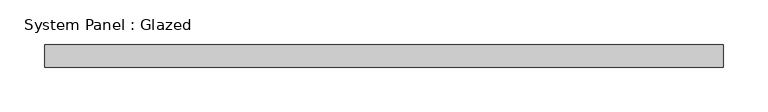
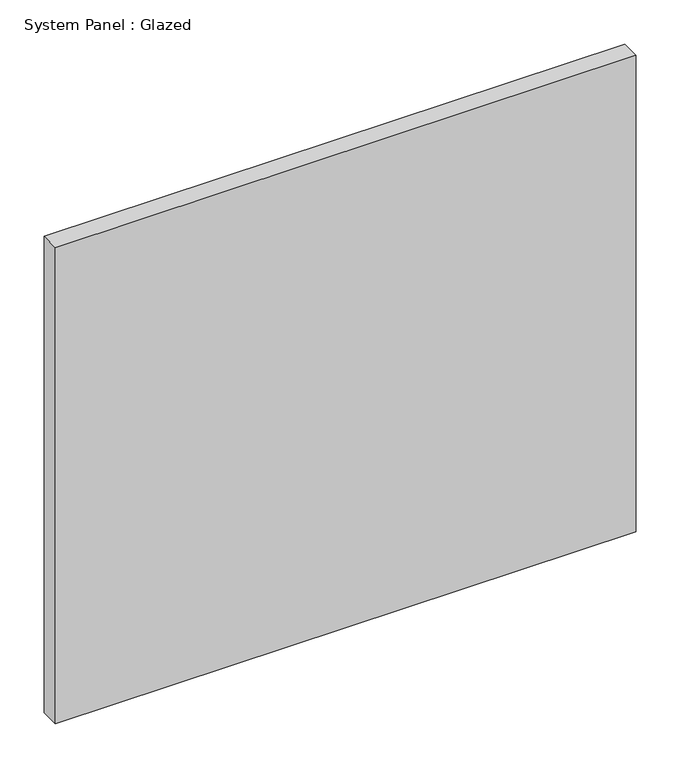
"""IFC4 building model written with IfcOpenShell, lengths in millimetres: plate geometry, System Panel : Glazed."""

from ifc_helpers import new_model, si_unit, origin, origin_with_axes, place, context, project, spatial, polyline, outline, extrude, source, transform, mapped, element, save


def system_panel_glazed_55f8bac4(model_context):
    return source(origin(), model_context, "Body", "SweptSolid", [
        extrude(outline(polyline([(381.0, 19.05), (-381.0, 19.05), (-381.0, 44.45), (381.0, 44.45), (381.0, 19.05)])), origin_with_axes(), (0.0, 0.0, 1.0), 660.4),
    ])


if __name__ == "__main__":
    model = new_model("IFC4")
    model_context = context("Model", 3, world=origin())
    ifc_project = project(units=[si_unit("LENGTHUNIT", "METRE", prefix="MILLI")], contexts=[model_context])
    site = spatial("IfcSite", under=ifc_project)
    building = spatial("IfcBuilding", under=site)
    placement = place(None, origin())
    system_panel_glazed_shape = system_panel_glazed_55f8bac4(model_context)
    element("IfcPlate", 1, ObjectType="System Panel : Glazed", at=placement, inside=building, context=model_context, shape_type="MappedRepresentation", body=[
        mapped(system_panel_glazed_shape, transform((0.0, 0.0, 0.0), x_axis=(1.0, 0.0, 0.0), y_axis=(0.0, 1.0, 0.0), z_axis=(0.0, 0.0, 1.0))),
    ])
    save(model, "model.ifc")

# Revit data of these elements
# Type "System Panel : Glazed"
#   Construction Type Id = "GSP4R"
#   Analytic Construction = "1/8 in Pilkington single glazing"
#   Visual Light Transmittance = 0.9
#   Solar Heat Gain Coefficient = 0.86
#   Heat Transfer Coefficient (U) = 1.18115 BTU/(h·ft²·°F)
# Element 1 (IfcPlate, "System Panel : Glazed")
#   Materials on its faces: "Glass"
# Materials
#   "Glass": class "Glass", colour RGB 0 128 192, transparency 0.75, Description = "Soda Lime Glass", Cost = 0
